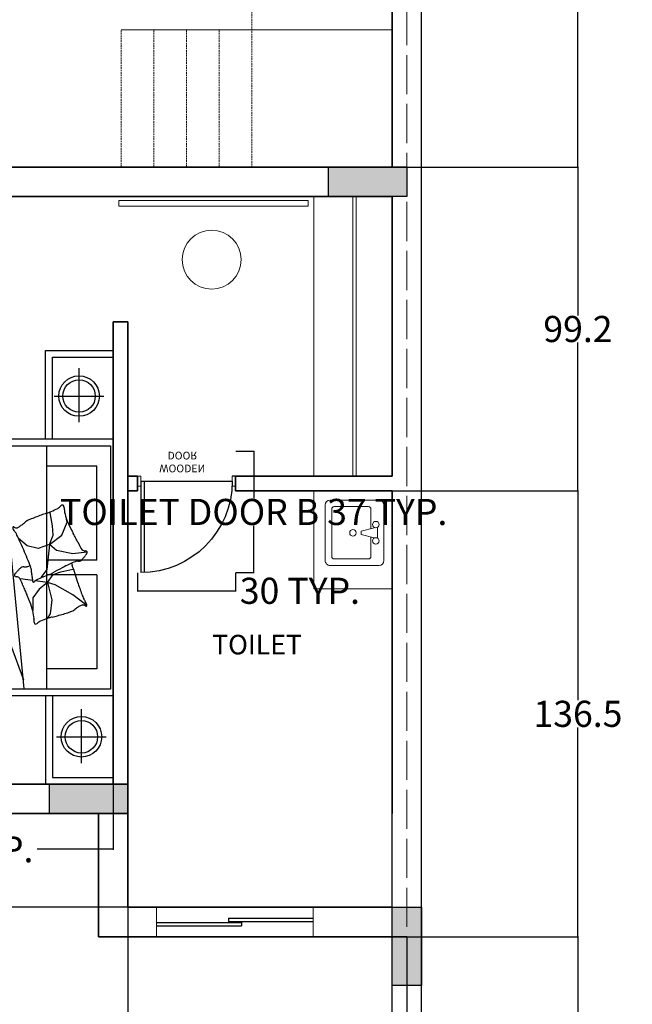
# Model space of a CAD drawing. Units: inches. Extents: x -48 to 50072, y 0 to 21068.
# Tile 64 of 75: x 1176 to 1363, y 501 to 803. Entities that reach past the tile are written whole.
import ezdxf

# ---------------------------------------------------------------- set-up
doc = ezdxf.new("R2010")
doc.units = ezdxf.units.IN
doc.header["$MEASUREMENT"] = 0
doc.linetypes.add('ACAD_ISO02W100', pattern=[15, 12, -3])
doc.linetypes.add('DASHED', pattern=[0.75, 0.5, -0.25])
for name, color, linetype, lineweight in [('A-ANNO-DIMS', 2, 'Continuous', 18), ('A-AREA-IDEN', 7, 'Continuous', 18), ('A-COLS', 1, 'Continuous', 35), ('A-DOOR', 4, 'Continuous', 18), ('A-FLOR-CASE', 9, 'Continuous', 18), ('A-FLOR-FIXT', 4, 'Continuous', 18), ('A-FLOR-STRS', 7, 'Continuous', 18), ('A-FLOR-STRS-HIDN', 8, 'DASHED', 13), ('A-GLAZ', 4, 'Continuous', 18), ('A-WALL', 7, 'Continuous', 35), ('C-PROP', 7, 'Continuous', 25), ('C-PROP-REF', 32, 'ACAD_ISO02W100', 13), ('FURNITURE', 44, 'Continuous', 18)]:
    doc.layers.add(name, color=color, linetype=linetype, lineweight=lineweight)
doc.layers.add('Layer3', color=176, linetype='Continuous')
doc.styles.get("Standard").update_dxf_attribs({"font": 'arial.ttf'})
doc.dimstyles.get("Standard").update_dxf_attribs({"dimtxt": 8, "dimasz": 0.18, "dimexe": 0.18, "dimexo": 0.0625, "dimgap": 0.09, "dimtad": 0, "dimtih": 1, "dimtoh": 1, "dimdec": 1, "dimzin": 0, "dimdsep": 46, "dimlunit": 4, "dimtxsty": 'Standard', "dimblk": 'ARCHTICK', "dimcen": 0.09, "dimadec": 0, "dimazin": 0, "dimtfac": 1, "dimtdec": 1, "dimtofl": 0, "dimtmove": 0, "dimatfit": 3, "dimldrblk": 'ARCHTICK', "dimfxl": 1, "dimtolj": 1, "dimtzin": 0, "dimarcsym": 0})

# ---------------------------------------------------------------- blocks, each defined once
blk = doc.blocks.new('bnniku')
at = {"layer": 'Defpoints'}
h = blk.add_hatch(color=256, dxfattribs=at)
h.dxf.hatch_style = 1
h.paths.add_polyline_path([(767.55, 1114.04), (758.55, 1114.04), (758.55, 1090.04), (767.55, 1090.04)])
for p, q in [((758.55, 1114.04), (767.55, 1114.04)), ((758.55, 1090.04), (758.55, 1114.04)), ((767.55, 1114.04), (767.55, 1090.04)), ((767.55, 1090.04), (758.55, 1090.04))]:
    blk.add_line(p, q, dxfattribs=at)
blk = doc.blocks.new('gthyerhy')
at = {"layer": 'Defpoints'}
for p, q in [((665.59, 603.33), (665.59, 631.33)), ((666.59, 603.33), (666.59, 631.32)), ((665.59, 603.33), (693.59, 603.33))]:
    blk.add_line(p, q, dxfattribs=at)
blk.add_arc((665.59, 603.33), 28, 0, 90, dxfattribs=at)
at = {"insert": (674.82, 600.63), "char_height": 2.3647, "attachment_point": 1}
blk.add_mtext_dynamic_manual_height_columns('\\pxqc;WOODEN ^JDOOR', width=6.8949, gutter_width=11.82, heights=[0], dxfattribs=at)
blk = doc.blocks.new('gfhdr6777ju')
for p, q in [((466.52, 596.57), (467.52, 596.57)), ((467.52, 593.57), (467.52, 596.57)), ((495.52, 593.57), (495.52, 596.57)), ((466.52, 593.57), (467.52, 593.57)), ((495.52, 593.57), (496.52, 593.57))]:
    blk.add_line(p, q)
at = {"layer": 'Defpoints'}
blk.add_line((496.52, 596.57), (495.52, 596.57), dxfattribs=at)
at = {"layer": 'Defpoints', "xscale": -1, "rotation": 180}
blk.add_blockref('gthyerhy', (-198.07, 1198.41), dxfattribs=at)
blk = doc.blocks.new('windom')
for p, q in [((48.52, 1025.77), (48.52, 1034.77)), ((96.52, 1025.77), (96.52, 1034.77))]:
    blk.add_line(p, q)
at = {"layer": 'Defpoints'}
for p, q in [((70.52, 1031.47), (96.52, 1031.47)), ((70.52, 1031.47), (70.52, 1030.47)), ((48.52, 1030.07), (74.52, 1030.07)), ((48.52, 1029.07), (74.52, 1029.07)), ((70.52, 1030.47), (96.52, 1030.47)), ((74.52, 1030.07), (74.52, 1029.07))]:
    blk.add_line(p, q, dxfattribs=at)
at = {"layer": 'Layer3'}
for p, q in [((48.52, 1034.77), (96.52, 1034.77)), ((48.52, 1025.77), (96.52, 1025.77))]:
    blk.add_line(p, q, dxfattribs=at)
blk = doc.blocks.new('nhrygfdu7yu')
at = {"layer": 'Defpoints'}
for p, q in [((1019.17, 828.61), (845.97, 828.61)), ((845.97, 801.61), (845.97, 828.61)), ((848.67, 804.31), (848.67, 828.61)), ((881.27, 716.83), (881.27, 828.61)), ((884.03, 719.53), (884.03, 827.53)), ((884.03, 827.53), (981.17, 827.53)), ((981.17, 827.53), (981.17, 719.53)), ((983.87, 828.61), (983.87, 716.83)), ((1000.24, 805.98), (1000.24, 825.78)), ((1016.47, 804.31), (1016.47, 828.61)), ((1019.17, 801.61), (1019.17, 828.61)), ((864.18, 805.04), (864.18, 824.84)), ((892.12, 822.13), (892.12, 801.97)), ((929.67, 822.13), (892.12, 822.13)), ((929.67, 822.13), (929.67, 801.78)), ((935.52, 822.13), (935.52, 801.78)), ((935.52, 822.13), (973.07, 822.13)), ((973.07, 822.13), (973.07, 801.97)), ((926.47, 818.07), (927.21, 812.5)), ((947.88, 818.06), (943.61, 812.45)), ((874.65, 814.99), (853.09, 814.99)), ((1010.72, 815.93), (989.15, 815.93)), ((914.58, 810.18), (913.28, 809.99)), ((919.69, 808.14), (914.58, 810.18)), ((927.21, 812.5), (925.82, 805.91)), ((934.43, 807.75), (933.36, 812.55)), ((943.61, 812.45), (939.55, 805.41)), ((923.4, 803.12), (919.69, 808.14)), ((935.49, 804.66), (934.43, 807.75)), ((881.07, 804.31), (848.67, 804.31)), ((881.07, 804.31), (881.07, 804.31)), ((910.77, 803.49), (910.59, 803.15)), ((916.07, 804.42), (910.77, 803.49)), ((919.78, 804.61), (916.07, 804.42)), ((923.4, 803.12), (919.78, 804.61)), ((925.82, 805.91), (923.4, 803.12)), ((923.4, 803.12), (925.08, 798.67)), ((923.4, 803.12), (933.44, 802.1)), ((933.44, 802.1), (936.13, 800.15)), ((935.45, 803.17), (936.69, 800.13)), ((938.59, 802.42), (935.49, 804.66)), ((938.59, 802.42), (937.95, 797.34)), ((939.55, 805.41), (938.59, 802.42)), ((938.59, 802.42), (945.53, 804.13)), ((938.59, 802.42), (941.26, 799.01)), ((945.53, 804.13), (951.08, 803.38)), ((951.08, 803.38), (953.02, 802.3)), ((984.07, 804.31), (1016.47, 804.31)), ((984.07, 804.31), (984.07, 804.31)), ((881.07, 801.61), (845.97, 801.61)), ((884.06, 801.97), (981.18, 801.97)), ((925.08, 798.67), (923.96, 794.21)), ((936.13, 800.15), (936.78, 799.69)), ((936.69, 800.13), (937.65, 797.78)), ((941.26, 799.01), (944.78, 796.45)), ((984.07, 801.61), (1019.17, 801.61)), ((923.96, 794.21), (921.07, 790.83)), ((937.86, 796.54), (937.22, 791.44)), ((944.78, 796.45), (949.8, 796.45)), ((981.13, 793.06), (883.98, 783.7)), ((906.36, 766.47), (977.44, 792.73)), ((976.41, 779.36), (976.41, 779.36)), ((978.98, 779.36), (978.98, 779.36)), ((962.27, 776.79), (962.27, 776.79)), ((964.84, 776.79), (964.84, 776.79)), ((967.41, 776.79), (967.41, 776.79)), ((969.98, 776.79), (969.98, 776.79)), ((972.55, 776.79), (972.55, 776.79)), ((975.13, 776.79), (975.13, 776.79)), ((977.7, 776.79), (977.7, 776.79)), ((980.27, 776.79), (980.27, 776.79)), ((941.69, 771.64), (941.69, 771.64)), ((944.27, 771.64), (944.27, 771.64)), ((946.84, 771.64), (946.84, 771.64)), ((949.41, 771.64), (949.41, 771.64)), ((950.69, 774.21), (950.69, 774.21)), ((951.98, 771.64), (951.98, 771.64)), ((953.27, 774.21), (953.27, 774.21)), ((954.55, 771.64), (954.55, 771.64)), ((955.84, 774.21), (955.84, 774.21)), ((958.41, 774.21), (958.41, 774.21)), ((960.98, 774.21), (960.98, 774.21)), ((963.55, 774.21), (963.55, 774.21)), ((966.13, 774.21), (966.13, 774.21)), ((968.7, 774.21), (968.7, 774.21)), ((935.26, 769.07), (935.26, 769.07)), ((937.84, 769.07), (937.84, 769.07)), ((940.41, 769.07), (940.41, 769.07)), ((942.98, 769.07), (942.98, 769.07)), ((924.98, 763.93), (924.98, 763.93)), ((927.55, 763.93), (927.55, 763.93)), ((928.83, 766.5), (928.83, 766.5)), ((930.12, 763.93), (930.12, 763.93)), ((931.41, 766.5), (931.41, 766.5)), ((933.98, 766.5), (933.98, 766.5)), ((936.55, 766.5), (936.55, 766.5)), ((963.55, 763.93), (963.55, 763.93)), ((966.13, 763.93), (966.13, 763.93)), ((968.7, 763.93), (968.7, 763.93)), ((971.27, 763.93), (971.27, 763.93)), ((973.84, 763.93), (973.84, 763.93)), ((975.13, 766.5), (975.13, 766.5)), ((976.41, 763.93), (976.41, 763.93)), ((977.7, 766.5), (977.7, 766.5)), ((978.98, 763.93), (978.98, 763.93)), ((980.27, 766.5), (980.27, 766.5)), ((921.12, 761.35), (921.12, 761.35)), ((923.69, 761.35), (923.69, 761.35)), ((954.55, 761.35), (954.55, 761.35)), ((957.12, 761.35), (957.12, 761.35)), ((959.7, 761.35), (959.7, 761.35)), ((962.27, 761.35), (962.27, 761.35)), ((964.84, 761.35), (964.84, 761.35)), ((967.41, 761.35), (967.41, 761.35)), ((969.98, 761.35), (969.98, 761.35)), ((972.55, 761.35), (972.55, 761.35)), ((975.13, 761.35), (975.13, 761.35)), ((913.4, 756.21), (913.4, 756.21)), ((915.98, 756.21), (915.98, 756.21)), ((917.26, 758.78), (917.26, 758.78)), ((919.83, 758.78), (919.83, 758.78)), ((941.69, 756.21), (941.69, 756.21)), ((944.27, 756.21), (944.27, 756.21)), ((945.55, 758.78), (945.55, 758.78)), ((946.84, 756.21), (946.84, 756.21)), ((948.12, 758.78), (948.12, 758.78)), ((949.41, 756.21), (949.41, 756.21)), ((950.69, 758.78), (950.69, 758.78)), ((951.98, 756.21), (951.98, 756.21)), ((953.27, 758.78), (953.27, 758.78)), ((954.55, 756.21), (954.55, 756.21)), ((955.84, 758.78), (955.84, 758.78)), ((957.12, 756.21), (957.12, 756.21)), ((958.41, 758.78), (958.41, 758.78)), ((960.98, 758.78), (960.98, 758.78)), ((963.55, 758.78), (963.55, 758.78)), ((980.27, 756.21), (980.27, 756.21)), ((905.69, 751.07), (905.69, 751.07)), ((908.26, 751.07), (908.26, 751.07)), ((909.55, 753.64), (909.55, 753.64)), ((912.12, 753.64), (912.12, 753.64)), ((931.41, 751.07), (931.41, 751.07)), ((933.98, 751.07), (933.98, 751.07)), ((935.26, 753.64), (935.26, 753.64)), ((936.55, 751.07), (936.55, 751.07)), ((937.84, 753.64), (937.84, 753.64)), ((939.12, 751.07), (939.12, 751.07)), ((940.41, 753.64), (940.41, 753.64)), ((941.69, 751.07), (941.69, 751.07)), ((942.98, 753.64), (942.98, 753.64)), ((944.27, 751.07), (944.27, 751.07)), ((945.55, 753.64), (945.55, 753.64)), ((948.12, 753.64), (948.12, 753.64)), ((969.98, 751.07), (969.98, 751.07)), ((972.55, 751.07), (972.55, 751.07)), ((975.13, 751.07), (975.13, 751.07)), ((976.41, 753.64), (976.41, 753.64)), ((977.7, 751.07), (977.7, 751.07)), ((978.98, 753.64), (978.98, 753.64)), ((980.27, 751.07), (980.27, 751.07)), ((904.4, 748.5), (904.4, 748.5)), ((927.55, 748.5), (927.55, 748.5)), ((930.12, 748.5), (930.12, 748.5)), ((932.69, 748.5), (932.69, 748.5)), ((935.26, 748.5), (935.26, 748.5)), ((937.84, 748.5), (937.84, 748.5)), ((940.41, 748.5), (940.41, 748.5)), ((966.13, 748.5), (966.13, 748.5)), ((968.7, 748.5), (968.7, 748.5)), ((971.27, 748.5), (971.27, 748.5)), ((973.84, 748.5), (973.84, 748.5)), ((976.41, 748.5), (976.41, 748.5)), ((978.98, 748.5), (978.98, 748.5)), ((896.69, 743.35), (896.69, 743.35)), ((899.26, 743.35), (899.26, 743.35)), ((900.55, 745.92), (900.55, 745.92)), ((903.12, 745.92), (903.12, 745.92)), ((919.83, 743.35), (919.83, 743.35)), ((922.41, 743.35), (922.41, 743.35)), ((923.69, 745.92), (923.69, 745.92)), ((924.98, 743.35), (924.98, 743.35)), ((926.26, 745.92), (926.26, 745.92)), ((927.55, 743.35), (927.55, 743.35)), ((928.83, 745.92), (928.83, 745.92)), ((930.12, 743.35), (930.12, 743.35)), ((931.41, 745.92), (931.41, 745.92)), ((932.69, 743.35), (932.69, 743.35)), ((933.98, 745.92), (933.98, 745.92)), ((960.98, 743.35), (960.98, 743.35)), ((962.27, 745.92), (962.27, 745.92)), ((963.55, 743.35), (963.55, 743.35)), ((964.84, 745.92), (964.84, 745.92)), ((966.13, 743.35), (966.13, 743.35)), ((967.41, 745.92), (967.41, 745.92)), ((968.7, 743.35), (968.7, 743.35)), ((969.98, 745.92), (969.98, 745.92)), ((971.27, 743.35), (971.27, 743.35)), ((972.55, 745.92), (972.55, 745.92)), ((973.84, 743.35), (973.84, 743.35)), ((975.13, 745.92), (975.13, 745.92)), ((977.7, 745.92), (977.7, 745.92)), ((895.4, 740.78), (895.4, 740.78)), ((915.98, 740.78), (915.98, 740.78)), ((918.55, 740.78), (918.55, 740.78)), ((921.12, 740.78), (921.12, 740.78)), ((923.69, 740.78), (923.69, 740.78)), ((926.26, 740.78), (926.26, 740.78)), ((928.83, 740.78), (928.83, 740.78)), ((957.12, 740.78), (957.12, 740.78)), ((959.7, 740.78), (959.7, 740.78)), ((962.27, 740.78), (962.27, 740.78)), ((964.84, 740.78), (964.84, 740.78)), ((967.41, 740.78), (967.41, 740.78)), ((969.98, 740.78), (969.98, 740.78)), ((887.69, 735.64), (887.69, 735.64)), ((890.26, 735.64), (890.26, 735.64)), ((891.54, 738.21), (891.54, 738.21)), ((894.12, 738.21), (894.12, 738.21)), ((910.83, 735.64), (910.83, 735.64)), ((913.4, 735.64), (913.4, 735.64)), ((914.69, 738.21), (914.69, 738.21)), ((915.98, 735.64), (915.98, 735.64)), ((917.26, 738.21), (917.26, 738.21)), ((918.55, 735.64), (918.55, 735.64)), ((919.83, 738.21), (919.83, 738.21)), ((921.12, 735.64), (921.12, 735.64)), ((922.41, 738.21), (922.41, 738.21)), ((924.98, 738.21), (924.98, 738.21)), ((951.98, 735.64), (951.98, 735.64)), ((954.55, 735.64), (954.55, 735.64)), ((955.84, 738.21), (955.84, 738.21)), ((957.12, 735.64), (957.12, 735.64)), ((958.41, 738.21), (958.41, 738.21)), ((959.7, 735.64), (959.7, 735.64)), ((960.98, 738.21), (960.98, 738.21)), ((962.27, 735.64), (962.27, 735.64)), ((963.55, 738.21), (963.55, 738.21)), ((964.84, 735.64), (964.84, 735.64)), ((966.13, 738.21), (966.13, 738.21)), ((886.4, 733.07), (886.4, 733.07)), ((888.97, 733.07), (888.97, 733.07)), ((909.55, 733.07), (909.55, 733.07)), ((912.12, 733.07), (912.12, 733.07)), ((914.69, 733.07), (914.69, 733.07)), ((917.26, 733.07), (917.26, 733.07)), ((919.83, 733.07), (919.83, 733.07)), ((950.69, 733.07), (950.69, 733.07)), ((953.27, 733.07), (953.27, 733.07)), ((955.84, 733.07), (955.84, 733.07)), ((958.41, 733.07), (958.41, 733.07)), ((960.98, 733.07), (960.98, 733.07)), ((885.12, 730.49), (885.12, 730.49)), ((904.4, 727.92), (904.4, 727.92)), ((905.69, 730.49), (905.69, 730.49)), ((906.97, 727.92), (906.97, 727.92)), ((908.26, 730.49), (908.26, 730.49)), ((909.55, 727.92), (909.55, 727.92)), ((910.83, 730.49), (910.83, 730.49)), ((912.12, 727.92), (912.12, 727.92)), ((913.4, 730.49), (913.4, 730.49)), ((915.98, 730.49), (915.98, 730.49)), ((945.55, 727.92), (945.55, 727.92)), ((946.84, 730.49), (946.84, 730.49)), ((948.12, 727.92), (948.12, 727.92)), ((949.41, 730.49), (949.41, 730.49)), ((950.69, 727.92), (950.69, 727.92)), ((951.98, 730.49), (951.98, 730.49)), ((953.27, 727.92), (953.27, 727.92)), ((954.55, 730.49), (954.55, 730.49)), ((955.84, 727.92), (955.84, 727.92)), ((957.12, 730.49), (957.12, 730.49)), ((958.41, 727.92), (958.41, 727.92)), ((959.7, 730.49), (959.7, 730.49)), ((900.55, 725.35), (900.55, 725.35)), ((903.12, 725.35), (903.12, 725.35)), ((905.69, 725.35), (905.69, 725.35)), ((908.26, 725.35), (908.26, 725.35)), ((910.83, 725.35), (910.83, 725.35)), ((944.27, 725.35), (944.27, 725.35)), ((946.84, 725.35), (946.84, 725.35)), ((949.41, 725.35), (949.41, 725.35)), ((951.98, 725.35), (951.98, 725.35)), ((954.55, 725.35), (954.55, 725.35)), ((981.17, 719.53), (884.03, 719.53)), ((895.4, 720.21), (895.4, 720.21)), ((897.97, 720.21), (897.97, 720.21)), ((899.26, 722.78), (899.26, 722.78)), ((900.55, 720.21), (900.55, 720.21)), ((901.83, 722.78), (901.83, 722.78)), ((903.12, 720.21), (903.12, 720.21)), ((904.4, 722.78), (904.4, 722.78)), ((905.69, 720.21), (905.69, 720.21)), ((906.97, 722.78), (906.97, 722.78)), ((939.12, 720.21), (939.12, 720.21)), ((941.69, 720.21), (941.69, 720.21)), ((942.98, 722.78), (942.98, 722.78)), ((944.27, 720.21), (944.27, 720.21)), ((945.55, 722.78), (945.55, 722.78)), ((946.84, 720.21), (946.84, 720.21)), ((948.12, 722.78), (948.12, 722.78)), ((949.41, 720.21), (949.41, 720.21)), ((950.69, 722.78), (950.69, 722.78)), ((951.98, 720.21), (951.98, 720.21)), ((953.27, 722.78), (953.27, 722.78)), ((983.87, 716.83), (881.27, 716.83))]:
    blk.add_line(p, q, dxfattribs=at)
for centre, radius in [((864.18, 814.99), 8.1), ((1000.24, 815.93), 8.1), ((1000.24, 815.93), 6.48), ((864.18, 814.99), 6.48)]:
    blk.add_circle(centre, radius, dxfattribs=at)
for centre, radius, start, end in [((926.67, 817.58), 0.687, 51.1864, 183.2455), ((924.75, 815.18), 3.76, 45.8726, 51.1864), ((929.07, 819.63), 2.44, 225.8726, 232.4713), ((948.22, 814.9), 3.25, 110.3452, 128.5854), ((947.75, 816.16), 1.9, 86.0516, 110.3452), ((947.87, 817.82), 0.239, 13.2808, 86.0516), ((947.77, 817.8), 0.34, 306.5792, 13.2808), ((971.1, 717.04), 108.88, 116.4147, 117.4999), ((848.26, 964.34), 167.25, 296.4147, 297.2902), ((924.05, 817.43), 1.94, 297.2902, 3.2455), ((940.16, 834.08), 20.66, 232.4713, 233.7837), ((906.88, 788.64), 35.67, 52.7849, 53.7837), ((921.35, 807.68), 11.75, 46.4776, 52.7849), ((926.56, 813.17), 4.18, 35.8936, 46.4776), ((928.96, 814.91), 1.22, 351.9508, 35.8936), ((932.62, 814.39), 2.47, 171.9508, 202.4162), ((883.03, 974.91), 169.83, 286.6085, 289.0836), ((848.62, 1074.38), 275.09, 289.0836, 290.1287), ((927.73, 858.54), 45.2, 290.1287, 292.7069), ((943.53, 820.78), 4.28, 292.7069, 308.5854), ((951.77, 816.3), 4.17, 169.5926, 177.2714), ((948.44, 816.46), 0.826, 177.2714, 194.5709), ((949.69, 816.78), 2.12, 194.5709, 206.8179), ((948.43, 816.91), 0.765, 126.5792, 169.5926), ((964.76, 824.4), 19.01, 206.8179, 210.9056), ((957.44, 820.02), 10.47, 210.9056, 219.7005), ((905.47, 831.87), 23.22, 282.6252, 290.7486), ((901.77, 841.65), 33.68, 290.7486, 297.4921), ((771.78, 1091.44), 315.27, 297.4921, 297.8482), ((1072.97, 521.35), 329.5, 117.4999, 117.8482), ((980.52, 834.15), 54.29, 202.4162, 205.0529), ((929.77, 818.2), 6.29, 280.7366, 286.6085), ((1013.86, 849.73), 91.09, 205.0529, 207.0884), ((946.01, 810.53), 4.37, 26.0735, 39.7005), ((940.41, 807.79), 10.61, 17.8396, 26.0735), ((847.55, 777.91), 108.16, 15.2625, 17.8396), ((908.02, 808.45), 0.313, 121.6917, 179.0386), ((908.61, 808.44), 0.905, 179.0386, 229.4914), ((909.3, 806.38), 2.75, 103.0402, 121.6917), ((905.38, 804.66), 4.08, 26.3332, 49.4914), ((909.41, 805.91), 3.23, 86.6119, 103.0402), ((780.21, 742.7), 143.74, 25.1732, 26.3332), ((909.8, 812.53), 3.4, 266.6119, 282.6252), ((1008.01, 846.74), 84.52, 207.0884, 209.936), ((866.04, 782.95), 89, 13.841, 15.2625), ((901.51, 799.71), 9.71, 20.7081, 25.1732), ((883.04, 792.73), 29.45, 18.2369, 20.7081), ((924.73, 798.79), 11.57, 22.2355, 29.936), ((981.05, 811.29), 29.45, 193.841, 196.3122), ((962.1, 805.74), 9.71, 196.3122, 200.7773), ((1087.42, 853.29), 143.74, 200.7773, 201.9373), ((995.54, 829.8), 89, 198.2369, 199.6584), ((1013.59, 836.25), 108.16, 199.6584, 202.2355), ((957.87, 801.11), 4.08, 201.9373, 225.0955), ((954.35, 797.58), 0.905, 354.6428, 45.0955), ((923.29, 799.33), 10.61, 202.2355, 210.4694), ((993.31, 637.11), 169.83, 111.0043, 113.4795), ((880.68, 777.46), 54.29, 18.0203, 19.3448), ((929.96, 793.49), 2.47, 347.5549, 18.0203), ((934.7, 789.77), 6.29, 98.1216, 111.0043), ((934.31, 792.46), 3.58, 85.4882, 98.1216), ((934.9, 799.87), 3.85, 265.4882, 277.6784), ((934.12, 805.65), 9.69, 277.6784, 284.8807), ((939.32, 786.09), 10.56, 97.9822, 104.8807), ((938.8, 798.25), 1.24, 202.2355, 252.8133), ((938.1, 794.73), 1.83, 85.7407, 97.9822), ((938.28, 797.05), 0.497, 265.7407, 289.3799), ((938.36, 796.82), 0.252, 289.3799, 72.8133), ((1069.09, 504.93), 315.27, 113.0962, 113.4523), ((958.63, 763.95), 33.68, 106.3527, 113.0962), ((955.69, 773.98), 23.22, 98.2293, 106.3527), ((952.85, 793.6), 3.4, 82.216, 98.2293), ((953.75, 800.17), 3.23, 262.216, 278.6443), ((953.82, 799.69), 2.75, 278.6443, 297.2959), ((954.94, 797.53), 0.313, 297.2959, 354.6428), ((917.92, 796.17), 4.37, 210.4694, 224.0964), ((907.26, 785.84), 10.47, 35.3015, 44.0964), ((900.29, 780.91), 19.01, 31.2138, 35.3015), ((914.73, 789.66), 2.12, 18.9668, 31.2138), ((915.96, 790.08), 0.826, 1.6673, 18.9668), ((939.83, 749.71), 45.2, 114.5246, 117.1028), ((1035.25, 540.56), 275.09, 113.4795, 114.5246), ((933.57, 792.7), 1.22, 167.5549, 211.4977), ((936.09, 794.24), 4.18, 211.4977, 222.0817), ((941.71, 799.32), 11.75, 222.0817, 228.389), ((957.59, 817.2), 35.67, 228.389, 229.3878), ((938.27, 789.81), 1.94, 112.8944, 178.8496), ((1002.58, 637.52), 167.25, 112.0188, 112.8944), ((899.06, 893.51), 108.88, 292.0188, 293.104), ((812.48, 1096.43), 329.5, 293.104, 293.4523), ((916.73, 788.79), 0.34, 130.9751, 197.6767), ((916.63, 788.76), 0.239, 197.6767, 270.4475), ((916, 789.63), 0.765, 310.9751, 353.9885), ((916.62, 790.42), 1.9, 270.4475, 294.7411), ((912.62, 789.98), 4.17, 353.9885, 1.6673), ((916.05, 791.65), 3.25, 294.7411, 312.9813), ((921.18, 786.14), 4.28, 117.1028, 132.9813), ((920.93, 774.44), 20.66, 48.0754, 49.3878), ((933.1, 787.99), 2.44, 41.4767, 48.0754), ((937.75, 792.1), 3.76, 221.4767, 226.7905), ((935.64, 789.86), 0.687, 226.7905, 358.8496)]:
    blk.add_arc(centre, radius, start, end, dxfattribs=at)
blk.add_ellipse((874.1, 762.91), major_axis=(32.71, 0), ratio=0.667085, start_param=0.16392, end_param=1.263761, dxfattribs=at)
blk = doc.blocks.new('A$C329C6BD7')
at = {"linetype": 'ByBlock'}
for p, q in [((0, 0.4191), (0, 0.0381)), ((0.4699, 0.4572), (0.0381, 0.4572)), ((0.2159, 0.4064), (0.2921, 0.4064)), ((0.508, 0.0381), (0.508, 0.4191)), ((0.0508, 0.0698), (0.0508, 0.3365)), ((0.0698, 0.3556), (0.2223, 0.3556)), ((0.2159, 0.381), (0.2413, 0.2794)), ((0.2667, 0.2794), (0.2921, 0.381)), ((0.2858, 0.3556), (0.4382, 0.3556)), ((0.4572, 0.3365), (0.4572, 0.0698)), ((0.2413, 0.2794), (0.2667, 0.2794)), ((0.4382, 0.0508), (0.0698, 0.0508)), ((0.0381, 0), (0.4699, 0))]:
    blk.add_line(p, q, dxfattribs=at)
for centre in [(0.1905, 0.3937), (0.3175, 0.3937), (0.254, 0.2159)]:
    blk.add_circle(centre, 0.0254, dxfattribs=at)
for centre, radius, start, end in [((0.0381, 0.4191), 0.0381, 90, 180), ((0.4699, 0.4191), 0.0381, 0, 90), ((0.0698, 0.3365), 0.0191, 90, 180), ((0.4382, 0.3365), 0.0191, 0, 90), ((0.0381, 0.0381), 0.0381, 180, 270), ((0.0698, 0.0698), 0.0191, 180, 270), ((0.4382, 0.0698), 0.0191, 270, 0), ((0.4699, 0.0381), 0.0381, 270, 0)]:
    blk.add_arc(centre, radius, start, end, dxfattribs=at)
blk = doc.blocks.new('_ArchTick')
at = {"color": 0, "linetype": 'ByBlock', "const_width": 0.15}
blk.add_lwpolyline([(-0.5, -0.5), (0.5, 0.5)], dxfattribs=at)
blk = doc.blocks.new('*D70')
at = {"layer": 'A-ANNO-DIMS', "color": 0, "lineweight": -2, "transparency": 16777216}
for p, q in [((1241.82, 670.4), (1247.51, 670.4)), ((1247.33, 670.4), (1247.33, 656.06)), ((1247.33, 633.26), (1247.33, 647.6)), ((1241.82, 633.26), (1247.51, 633.26))]:
    blk.add_line(p, q, dxfattribs=at)
at = {"layer": 'Defpoints', "color": 0, "transparency": 16777216}
for p in [(1241.76, 670.4), (1247.33, 670.4), (1241.76, 633.26)]:
    blk.add_point(p, dxfattribs=at)
at = {"layer": 'A-ANNO-DIMS', "color": 0, "lineweight": -2, "transparency": 16777216, "xscale": 0.18, "yscale": 0.18, "zscale": 0.18}
for p, rotation in [((1247.33, 670.4), 90), ((1247.33, 633.26), 270)]:
    blk.add_blockref('_ArchTick', p, dxfattribs=dict(at, rotation=rotation))
at = {"layer": 'A-ANNO-DIMS', "color": 0, "transparency": 16777216, "insert": (1247.33, 651.83), "char_height": 8, "attachment_point": 5}
blk.add_mtext('\\A1;TOILET DOOR B 37 TYP.', dxfattribs=at)
blk = doc.blocks.new('*D71')
at = {"layer": 'A-ANNO-DIMS', "color": 0, "lineweight": -2, "transparency": 16777216}
for p, q in [((1211.76, 633.2), (1211.76, 627.51)), ((1241.76, 633.2), (1241.76, 627.51)), ((1211.76, 627.69), (1241.76, 627.69)), ((1241.76, 627.69), (1241.94, 627.69))]:
    blk.add_line(p, q, dxfattribs=at)
at = {"layer": 'Defpoints', "color": 0, "transparency": 16777216}
for p in [(1211.76, 633.26), (1241.76, 633.26), (1241.76, 627.69)]:
    blk.add_point(p, dxfattribs=at)
at = {"layer": 'A-ANNO-DIMS', "color": 0, "lineweight": -2, "transparency": 16777216, "xscale": 0.18, "yscale": 0.18, "zscale": 0.18, "rotation": 180}
blk.add_blockref('_ArchTick', (1211.76, 627.69), dxfattribs=at)
at = {"layer": 'A-ANNO-DIMS', "color": 0, "lineweight": -2, "transparency": 16777216, "xscale": 0.18, "yscale": 0.18, "zscale": 0.18}
blk.add_blockref('_ArchTick', (1241.76, 627.69), dxfattribs=at)
at = {"layer": 'A-ANNO-DIMS', "color": 0, "transparency": 16777216, "insert": (1261.5, 627.69), "char_height": 8, "attachment_point": 5}
blk.add_mtext('\\A1;30 TYP.', dxfattribs=at)
blk = doc.blocks.new('*D73')
at = {"layer": 'A-ANNO-DIMS', "color": 0, "lineweight": -2, "transparency": 16777216}
for p, q in [((1118.53, 568.4), (1118.53, 548.36)), ((1204.26, 568.4), (1204.26, 548.36)), ((1118.53, 548.54), (1141.83, 548.54)), ((1204.26, 548.54), (1180.96, 548.54))]:
    blk.add_line(p, q, dxfattribs=at)
at = {"layer": 'Defpoints', "color": 0, "transparency": 16777216}
for p in [(1118.53, 568.46), (1204.26, 568.46), (1204.26, 548.54)]:
    blk.add_point(p, dxfattribs=at)
at = {"layer": 'A-ANNO-DIMS', "color": 0, "lineweight": -2, "transparency": 16777216, "xscale": 0.18, "yscale": 0.18, "zscale": 0.18, "rotation": 180}
blk.add_blockref('_ArchTick', (1118.53, 548.54), dxfattribs=at)
at = {"layer": 'A-ANNO-DIMS', "color": 0, "lineweight": -2, "transparency": 16777216, "xscale": 0.18, "yscale": 0.18, "zscale": 0.18}
blk.add_blockref('_ArchTick', (1204.26, 548.54), dxfattribs=at)
at = {"layer": 'A-ANNO-DIMS', "color": 0, "transparency": 16777216, "insert": (1161.4, 548.54), "char_height": 8, "attachment_point": 5}
blk.add_mtext('\\A1;86 TYP.', dxfattribs=at)
blk = doc.blocks.new('*D132')
at = {"layer": 'A-ANNO-DIMS', "color": 0, "lineweight": -2, "transparency": 16777216}
for p, q in [((1294.32, 521.76), (1346.89, 521.76)), ((1346.71, 521.76), (1346.71, 407.44)), ((1346.71, 284.76), (1346.71, 399.09)), ((1298.82, 284.76), (1346.89, 284.76))]:
    blk.add_line(p, q, dxfattribs=at)
at = {"layer": 'Defpoints', "color": 0, "transparency": 16777216}
for p in [(1294.26, 521.76), (1346.71, 521.76), (1298.76, 284.76)]:
    blk.add_point(p, dxfattribs=at)
at = {"layer": 'A-ANNO-DIMS', "color": 0, "lineweight": -2, "transparency": 16777216, "xscale": 0.18, "yscale": 0.18, "zscale": 0.18}
for p, rotation in [((1346.71, 521.76), 90), ((1346.71, 284.76), 270)]:
    blk.add_blockref('_ArchTick', p, dxfattribs=dict(at, rotation=rotation))
at = {"layer": 'A-ANNO-DIMS', "color": 0, "transparency": 16777216, "insert": (1346.71, 403.26), "char_height": 8, "attachment_point": 5}
blk.add_mtext('\\A1;237', dxfattribs=at)
blk = doc.blocks.new('*D134')
at = {"layer": 'A-ANNO-DIMS', "color": 0, "lineweight": -2, "transparency": 16777216}
for p, q in [((1294.32, 931.53), (1346.89, 931.53)), ((1346.71, 931.53), (1346.71, 848.67)), ((1346.71, 757.46), (1346.71, 840.32)), ((1294.32, 757.46), (1346.89, 757.46))]:
    blk.add_line(p, q, dxfattribs=at)
at = {"layer": 'Defpoints', "color": 0, "transparency": 16777216}
for p in [(1294.26, 931.53), (1294.26, 757.46), (1346.71, 757.46)]:
    blk.add_point(p, dxfattribs=at)
at = {"layer": 'A-ANNO-DIMS', "color": 0, "lineweight": -2, "transparency": 16777216, "xscale": 0.18, "yscale": 0.18, "zscale": 0.18}
for p, rotation in [((1346.71, 931.53), 90), ((1346.71, 757.46), 270)]:
    blk.add_blockref('_ArchTick', p, dxfattribs=dict(at, rotation=rotation))
at = {"layer": 'A-ANNO-DIMS', "color": 0, "transparency": 16777216, "insert": (1346.71, 844.5), "char_height": 8, "attachment_point": 5}
blk.add_mtext('\\A1;174.06', dxfattribs=at)
blk = doc.blocks.new('*D138')
at = {"layer": 'A-ANNO-DIMS', "color": 0, "lineweight": -2, "transparency": 16777216}
for p, q in [((1042.26, 559.4), (1042.26, 236.63)), ((1208.76, 559.4), (1208.76, 236.63)), ((1042.26, 236.81), (1112.27, 236.81)), ((1208.76, 236.81), (1138.75, 236.81))]:
    blk.add_line(p, q, dxfattribs=at)
at = {"layer": 'Defpoints', "color": 0, "transparency": 16777216}
for p in [(1042.26, 559.46), (1208.76, 559.46), (1208.76, 236.81)]:
    blk.add_point(p, dxfattribs=at)
at = {"layer": 'A-ANNO-DIMS', "color": 0, "lineweight": -2, "transparency": 16777216, "xscale": 0.18, "yscale": 0.18, "zscale": 0.18, "rotation": 180}
blk.add_blockref('_ArchTick', (1042.26, 236.81), dxfattribs=at)
at = {"layer": 'A-ANNO-DIMS', "color": 0, "lineweight": -2, "transparency": 16777216, "xscale": 0.18, "yscale": 0.18, "zscale": 0.18}
blk.add_blockref('_ArchTick', (1208.76, 236.81), dxfattribs=at)
at = {"layer": 'A-ANNO-DIMS', "color": 0, "transparency": 16777216, "insert": (1125.51, 236.81), "char_height": 8, "attachment_point": 5}
blk.add_mtext('\\A1;166.5', dxfattribs=at)
blk = doc.blocks.new('*D139')
at = {"layer": 'A-ANNO-DIMS', "color": 0, "lineweight": -2, "transparency": 16777216}
for p, q in [((1208.76, 530.7), (1208.76, 236.63)), ((1294.26, 521.7), (1294.26, 236.63)), ((1208.76, 236.81), (1241, 236.81)), ((1294.26, 236.81), (1262.03, 236.81))]:
    blk.add_line(p, q, dxfattribs=at)
at = {"layer": 'Defpoints', "color": 0, "transparency": 16777216}
for p in [(1208.76, 530.76), (1294.26, 521.76), (1294.26, 236.81)]:
    blk.add_point(p, dxfattribs=at)
at = {"layer": 'A-ANNO-DIMS', "color": 0, "lineweight": -2, "transparency": 16777216, "xscale": 0.18, "yscale": 0.18, "zscale": 0.18, "rotation": 180}
blk.add_blockref('_ArchTick', (1208.76, 236.81), dxfattribs=at)
at = {"layer": 'A-ANNO-DIMS', "color": 0, "lineweight": -2, "transparency": 16777216, "xscale": 0.18, "yscale": 0.18, "zscale": 0.18}
blk.add_blockref('_ArchTick', (1294.26, 236.81), dxfattribs=at)
at = {"layer": 'A-ANNO-DIMS', "color": 0, "transparency": 16777216, "insert": (1251.51, 236.81), "char_height": 8, "attachment_point": 5}
blk.add_mtext('\\A1;85.5', dxfattribs=at)
blk = doc.blocks.new('*D140')
at = {"layer": 'A-ANNO-DIMS', "color": 0, "lineweight": -2, "transparency": 16777216}
for p, q in [((1289.82, 658.26), (1346.89, 658.26)), ((1346.71, 658.26), (1346.71, 594.19)), ((1346.71, 521.76), (1346.71, 585.84)), ((1294.32, 521.76), (1346.89, 521.76))]:
    blk.add_line(p, q, dxfattribs=at)
at = {"layer": 'Defpoints', "color": 0, "transparency": 16777216}
for p in [(1289.76, 658.26), (1346.71, 658.26), (1294.26, 521.76)]:
    blk.add_point(p, dxfattribs=at)
at = {"layer": 'A-ANNO-DIMS', "color": 0, "lineweight": -2, "transparency": 16777216, "xscale": 0.18, "yscale": 0.18, "zscale": 0.18}
for p, rotation in [((1346.71, 658.26), 90), ((1346.71, 521.76), 270)]:
    blk.add_blockref('_ArchTick', p, dxfattribs=dict(at, rotation=rotation))
at = {"layer": 'A-ANNO-DIMS', "color": 0, "transparency": 16777216, "insert": (1346.71, 590.01), "char_height": 8, "attachment_point": 5}
blk.add_mtext('\\A1;136.5', dxfattribs=at)
blk = doc.blocks.new('*D141')
at = {"layer": 'A-ANNO-DIMS', "color": 0, "lineweight": -2, "transparency": 16777216}
for p, q in [((1294.32, 757.46), (1346.89, 757.46)), ((1346.71, 757.46), (1346.71, 712.04)), ((1346.71, 658.26), (1346.71, 703.69)), ((1289.82, 658.26), (1346.89, 658.26))]:
    blk.add_line(p, q, dxfattribs=at)
at = {"layer": 'Defpoints', "color": 0, "transparency": 16777216}
for p in [(1294.26, 757.46), (1346.71, 757.46), (1289.76, 658.26)]:
    blk.add_point(p, dxfattribs=at)
at = {"layer": 'A-ANNO-DIMS', "color": 0, "lineweight": -2, "transparency": 16777216, "xscale": 0.18, "yscale": 0.18, "zscale": 0.18}
for p, rotation in [((1346.71, 757.46), 90), ((1346.71, 658.26), 270)]:
    blk.add_blockref('_ArchTick', p, dxfattribs=dict(at, rotation=rotation))
at = {"layer": 'A-ANNO-DIMS', "color": 0, "transparency": 16777216, "insert": (1346.71, 707.86), "char_height": 8, "attachment_point": 5}
blk.add_mtext('\\A1;99.2', dxfattribs=at)
blk = doc.blocks.new('*D146')
at = {"layer": 'A-ANNO-DIMS', "color": 0, "lineweight": -2, "transparency": 16777216}
for p, q in [((1208.7, 559.46), (710.63, 559.46)), ((710.81, 559.46), (710.81, 549.29)), ((710.81, 530.76), (710.81, 540.94)), ((1208.7, 530.76), (710.63, 530.76))]:
    blk.add_line(p, q, dxfattribs=at)
at = {"layer": 'Defpoints', "color": 0, "transparency": 16777216}
for p in [(710.81, 559.46), (1208.76, 559.46), (1208.76, 530.76)]:
    blk.add_point(p, dxfattribs=at)
at = {"layer": 'A-ANNO-DIMS', "color": 0, "lineweight": -2, "transparency": 16777216, "xscale": 0.18, "yscale": 0.18, "zscale": 0.18}
for p, rotation in [((710.81, 559.46), 90), ((710.81, 530.76), 270)]:
    blk.add_blockref('_ArchTick', p, dxfattribs=dict(at, rotation=rotation))
at = {"layer": 'A-ANNO-DIMS', "color": 0, "transparency": 16777216, "insert": (710.81, 545.11), "char_height": 8, "attachment_point": 5}
blk.add_mtext('\\A1;28.7', dxfattribs=at)

msp = doc.modelspace()

# ---------------------------------------------------------------- linework, layer by layer
at = {"layer": 'A-FLOR-CASE'}
for p, q in [((1265.761, 662.764), (1265.761, 748.464)), ((1277.761, 662.764), (1277.761, 748.464)), ((1278.761, 662.764), (1278.761, 748.464)), ((1265.761, 628.264), (1265.761, 658.264)), ((1265.761, 628.264), (1289.761, 628.264))]:
    msp.add_line(p, q, dxfattribs=at)
at = {"layer": 'A-FLOR-STRS'}
msp.add_line((1289.761, 799.464), (1206.761, 799.464), dxfattribs=at)
at = {"layer": 'A-FLOR-STRS-HIDN'}
for p, q in [((1246.761, 839.527), (1246.761, 757.527)), ((1206.761, 757.527), (1206.761, 799.527)), ((1289.761, 799.527), (1206.761, 799.527)), ((1216.761, 757.527), (1216.761, 799.527)), ((1226.761, 757.527), (1226.761, 799.527)), ((1236.761, 757.527), (1236.761, 799.527))]:
    msp.add_line(p, q, dxfattribs=at)
at = {"layer": 'A-WALL'}
for p, q in [((1289.761, 757.464), (1289.761, 931.527)), ((1294.261, 757.464), (1042.261, 757.464)), ((1289.761, 748.464), (1042.261, 748.464)), ((1289.761, 662.764), (1289.761, 748.464)), ((1204.261, 568.464), (1204.261, 710.057)), ((1204.261, 710.057), (1208.761, 710.057)), ((1208.761, 662.764), (1208.761, 710.057)), ((1208.761, 662.764), (1211.761, 662.764)), ((1208.761, 530.764), (1208.761, 662.764)), ((1211.761, 658.264), (1211.761, 662.764)), ((1241.761, 662.764), (1289.761, 662.764)), ((1241.761, 658.264), (1241.761, 662.764)), ((1208.761, 658.264), (1211.761, 658.264)), ((1241.761, 658.264), (1289.761, 658.264)), ((1289.761, 559.464), (1289.761, 658.264)), ((1208.761, 568.464), (961.261, 568.464)), ((1208.761, 559.464), (961.261, 559.464)), ((1199.761, 521.764), (1199.761, 559.464)), ((1208.761, 530.764), (1208.761, 559.464)), ((1208.761, 530.764), (1289.761, 530.764)), ((1199.761, 521.764), (1294.261, 521.764))]:
    msp.add_line(p, q, dxfattribs=at)
at = {"layer": 'C-PROP'}
for p, q in [((1298.761, 284.764), (1298.761, 1241.464)), ((1289.761, 293.764), (1289.761, 559.464))]:
    msp.add_line(p, q, dxfattribs=at)
at = {"layer": 'C-PROP-REF'}
msp.add_line((1294.261, 284.764), (1294.261, 1236.964), dxfattribs=at)
at = {"layer": 'FURNITURE'}
msp.add_lwpolyline([(1205.976, 747.193), (1264.051, 747.193), (1264.051, 745.519), (1205.976, 745.519)], close=True, dxfattribs=at)
msp.add_circle((1234.459, 729.094), 9.039, dxfattribs=at)

# ---------------------------------------------------------------- block references
at = {"layer": 'A-COLS'}
for p, rotation in [((2384.298, -10.088), 90), ((94.724, 1327.016), 270)]:
    msp.add_blockref('bnniku', p, dxfattribs=dict(at, rotation=rotation))
msp.add_blockref('bnniku', (531.209, -583.273), dxfattribs=at)
at = {"layer": 'A-DOOR'}
msp.add_blockref('gfhdr6777ju', (745.244, 66.189), dxfattribs=at)
at = {"layer": 'A-FLOR-FIXT', "xscale": 39.38263526611686, "yscale": 39.38263526611686, "zscale": 39.38263526611686, "rotation": 270}
msp.add_blockref('A$C329C6BD7', (1269.254, 655.452), dxfattribs=at)
at = {"layer": 'A-GLAZ'}
msp.add_blockref('windom', (1169.078, -504.011), dxfattribs=at)
at = {"layer": 'FURNITURE', "xscale": 0.7669307891904348, "yscale": 0.7669307891904348, "zscale": 0.7669307891904348, "rotation": 270}
msp.add_blockref('nhrygfdu7yu', (568.778, 1350.095), dxfattribs=at)

# ---------------------------------------------------------------- texts
at = {"layer": 'A-AREA-IDEN', "insert": (1234.593, 614.207), "char_height": 6, "attachment_point": 1}
msp.add_mtext_dynamic_manual_height_columns('TOILET ', width=46.2236, gutter_width=30, heights=[0], dxfattribs=at)

# ---------------------------------------------------------------- dimensions: what is measured, and where the dimension line sits
at = {"layer": 'A-ANNO-DIMS'}
for base, p1, p2, override, picture, middle in [((1346.711, 757.464), (1294.261, 931.527), (1294.261, 757.464), {"dimdec": 2, "dimlfac": 1, "dimrnd": 0, "dimzin": 0, "dimdsep": 46, "dimlunit": 2}, '*D134', (1346.711, 844.496)), ((1346.711, 757.464), (1289.761, 658.264), (1294.261, 757.464), {"dimdec": 1, "dimlfac": 1, "dimrnd": 0, "dimzin": 0, "dimdsep": 46, "dimlunit": 2}, '*D141', (1346.711, 707.864)), ((1346.711, 658.264), (1294.261, 521.764), (1289.761, 658.264), {"dimdec": 1, "dimlfac": 1, "dimrnd": 0, "dimzin": 0, "dimdsep": 46, "dimlunit": 2}, '*D140', (1346.711, 590.014)), ((710.811, 559.464), (1208.761, 530.764), (1208.761, 559.464), {"dimdec": 1, "dimlfac": 1, "dimrnd": 0, "dimzin": 0, "dimdsep": 46, "dimlunit": 2}, '*D146', (710.811, 545.114)), ((1346.711, 521.764), (1298.761, 284.764), (1294.261, 521.764), {"dimdec": 0, "dimlfac": 1, "dimrnd": 0, "dimzin": 0, "dimdsep": 46, "dimlunit": 2}, '*D132', (1346.711, 403.264))]:
    dim = msp.add_linear_dim(base=base, p1=p1, p2=p2, angle=90, dimstyle='Standard', override=override, dxfattribs=at)
    dim.commit()
    dim.dimension.update_dxf_attribs({"geometry": picture, "text_midpoint": middle})
dim = msp.add_linear_dim(base=(1247.331, 670.4), p1=(1241.761, 633.264), p2=(1241.761, 670.4), angle=90, text='TOILET DOOR B <> TYP.', dimstyle='Standard', override={"dimdec": 0, "dimlfac": 1, "dimrnd": 0, "dimzin": 0, "dimdsep": 46, "dimlunit": 2}, dxfattribs=at)
dim.commit()
dim.dimension.update_dxf_attribs({"geometry": '*D70', "text_midpoint": (1247.331, 651.832)})
for base, p1, p2, picture, middle in [((1241.761, 627.694), (1211.761, 633.264), (1241.761, 633.264), '*D71', (1261.499, 627.694)), ((1204.261, 548.539), (1118.533, 568.464), (1204.261, 568.464), '*D73', (1161.397, 548.539))]:
    dim = msp.add_linear_dim(base=base, p1=p1, p2=p2, text='<> TYP.', dimstyle='Standard', override={"dimdec": 0, "dimlfac": 1, "dimrnd": 0, "dimzin": 0, "dimdsep": 46, "dimlunit": 2}, dxfattribs=at)
    dim.commit()
    dim.dimension.update_dxf_attribs({"geometry": picture, "text_midpoint": middle})
for base, p1, p2, picture, middle in [((1208.761, 236.814), (1042.261, 559.464), (1208.761, 559.464), '*D138', (1125.511, 236.814)), ((1294.261, 236.814), (1208.761, 530.764), (1294.261, 521.764), '*D139', (1251.511, 236.814))]:
    dim = msp.add_linear_dim(base=base, p1=p1, p2=p2, dimstyle='Standard', override={"dimdec": 1, "dimlfac": 1, "dimrnd": 0, "dimzin": 0, "dimdsep": 46, "dimlunit": 2}, dxfattribs=at)
    dim.commit()
    dim.dimension.update_dxf_attribs({"geometry": picture, "text_midpoint": middle})

doc.saveas('drawing.dxf')
